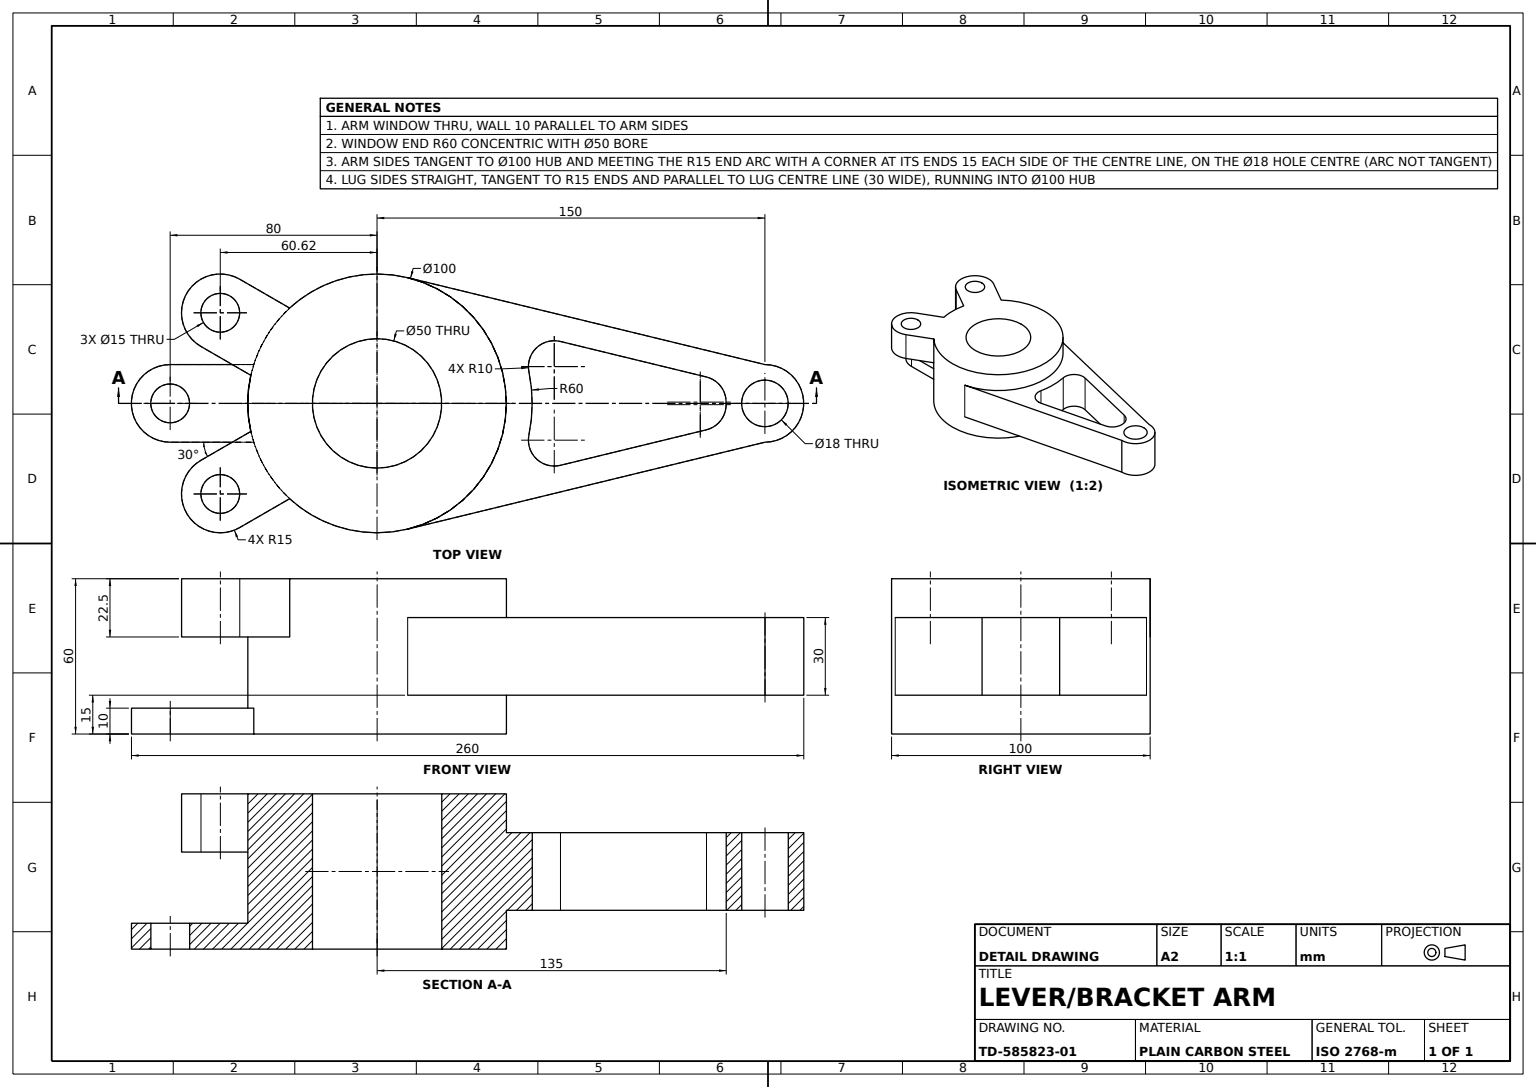
from build123d import *

# Parameters (mm, degrees)
HUB_SKETCH_R                = 50
HUB_SKETCH_R_2              = 25
HUB_100_BORE_50_DEPTH       = 60
LEVER_ARM_SKETCH_R          = 9
LEVER_ARM_DEPTH             = 15
ARM_LIGHTENING_WINDOW_DEPTH = 179.185296812
EAR_A_SKETCH_R              = 7.5
MOUNTING_EAR_A_DEPTH        = 22.5
MOUNTING_START              = -22.5
EAR_B_SKETCH_R              = 7.5
MOUNTING_EAR_B_DEPTH        = 22.5
ARM_WEB_SKETCH_R            = 7.5
ARM_WEB_10MM_DEPTH          = 10


with BuildPart() as part:
    # Hub Sketch → Hub Ø100 Bore Ø50 (new body)
    with BuildSketch(Plane(origin=(0, 0, 0), x_dir=(1, 0, 0), z_dir=(0, 1, 0))):
        with Locations(Location((0, 0, 0), (0, 0, 270))):
            Circle(HUB_SKETCH_R)
        with Locations(Location((0, 0, 0), (0, 0, 270))):
            Circle(HUB_SKETCH_R_2, mode=Mode.SUBTRACT)
    extrude(amount=HUB_100_BORE_50_DEPTH)

    # Lever Arm Sketch → Lever Arm (add, symmetric)
    with BuildSketch(Plane(origin=(0, 30, 0), x_dir=(1, 0, 0), z_dir=(0, 1, 0))):
        with BuildLine():
            Line((11.808098134, 48.585685325), (150, 15))
            ThreePointArc((150, 15), (165, 0), (150, -15))
            Line((150, -15), (11.808098134, -48.585685325))
            ThreePointArc((11.808098134, -48.585685325), (50, 0), (11.808098134, 48.585685325))
        make_face()
        with Locations(Location((150, 0, 0), (0, 0, 270))):
            Circle(LEVER_ARM_SKETCH_R, mode=Mode.SUBTRACT)
    extrude(amount=LEVER_ARM_DEPTH, both=True)

    # Arm Window Sketch → Arm Lightening Window (cut, through all)
    with BuildSketch(Plane(origin=(0, 45, 0), x_dir=(1, 0, 0), z_dir=(0, 1, 0))):
        with BuildLine():
            Line((127.366472028, 10.209677932), (70.90304943, 23.932354284))
            ThreePointArc((70.90304943, 23.932354284), (61.591288857, 21.405178334), (58.749796974, 12.184471902))
            ThreePointArc((58.749796974, 12.184471902), (60, 0), (58.749796974, -12.184471902))
            ThreePointArc((58.749796974, -12.184471902), (61.591288857, -21.405178334), (70.90304943, -23.932354284))
            Line((70.90304943, -23.932354284), (127.366472028, -10.209677932))
            ThreePointArc((127.366472028, -10.209677932), (132.927164163, -6.594751643), (135.002911441, -0.29552452))
            ThreePointArc((135.002911441, -0.29552452), (135, 0), (135.002911441, 0.29552452))
            ThreePointArc((135.002911441, 0.29552452), (132.927164163, 6.594751643), (127.366472028, 10.209677932))
        make_face()
    extrude(amount=-ARM_LIGHTENING_WINDOW_DEPTH, mode=Mode.SUBTRACT)

    # Ear A Sketch → Mounting Ear A (add)
    with BuildSketch(Plane(origin=(0, 60, 0), x_dir=(1, 0, 0), z_dir=(0, 1, 0))):
        with BuildLine():
            Line((-48.770060726, -10.836899613), (-68.121778265, -22.009618943))
            ThreePointArc((-68.121778265, -22.009618943), (-73.612159322, -42.5), (-53.121778265, -47.990381057))
            Line((-53.121778265, -47.990381057), (-33.644953635, -36.745431114))
            ThreePointArc((-33.644953635, -36.745431114), (-43.203476292, -24.956389512), (-48.770060726, -10.836899613))
        make_face()
        with Locations(Location((-60.621778265, -35, 0), (0, 0, 270))):
            Circle(EAR_A_SKETCH_R, mode=Mode.SUBTRACT)
    extrude(amount=-MOUNTING_EAR_A_DEPTH)

    # Ear B Sketch → Mounting Ear B (add)
    with BuildSketch(Plane(origin=(0, 60, 0), x_dir=(1, 0, 0), z_dir=(0, 1, 0)).offset(MOUNTING_START)):
        with BuildLine():
            Line((-33.806779105, 36.838861092), (-53.121778265, 47.990381057))
            ThreePointArc((-53.121778265, 47.990381057), (-73.612159322, 42.5), (-68.121778265, 22.009618943))
            Line((-68.121778265, 22.009618943), (-48.806779105, 10.858098979))
            ThreePointArc((-48.806779105, 10.858098979), (-43.301270189, 25), (-33.806779105, 36.838861092))
        make_face()
        with Locations(Location((-60.621778265, 35, 0), (0, 0, 270))):
            Circle(EAR_B_SKETCH_R, mode=Mode.SUBTRACT)
    extrude(amount=MOUNTING_EAR_B_DEPTH)

    # Arm Web Sketch → Arm Web 10mm (add)
    with BuildSketch(Plane(origin=(0, 0, 0), x_dir=(1, 0, 0), z_dir=(0, 1, 0))):
        with BuildLine():
            Line((-80, 15), (-50.661233673, 15))
            Line((-50.661233673, 15), (-43.043702026, 15))
            Line((-43.043702026, 15), (-43.043702026, -15))
            Line((-43.043702026, -15), (-80, -15))
            ThreePointArc((-80, -15), (-95, 0), (-80, 15))
        make_face()
        with Locations(Location((-80, 0, 0), (0, 0, 270))):
            Circle(ARM_WEB_SKETCH_R, mode=Mode.SUBTRACT)
    extrude(amount=ARM_WEB_10MM_DEPTH)


solid = part.part
